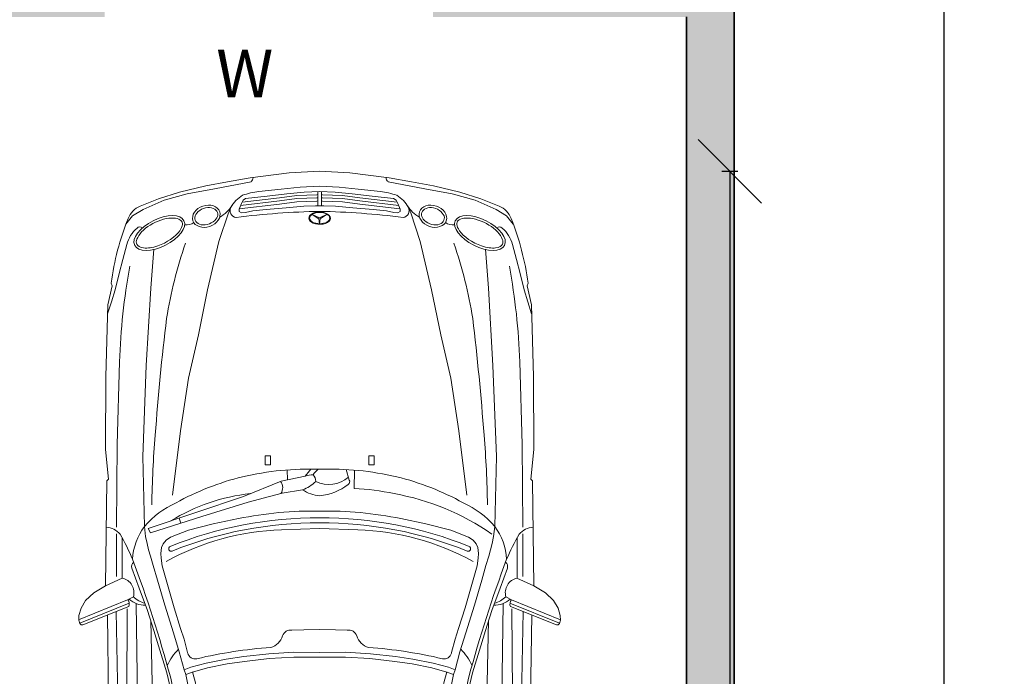
# Model space of a CAD drawing. Units: inches. Extents: x 2247 to 2713, y 588 to 1209.
# Tile 3 of 5: x 2574 to 2698, y 725 to 808. Entities that reach past the tile are written whole.
import ezdxf

# ---------------------------------------------------------------- set-up
doc = ezdxf.new("R2010")
doc.units = ezdxf.units.IN
for name, color, linetype, lineweight in [('0_Equip', 250, 'Continuous', 18), ('A-ANNO-DIMS', 2, 'Continuous', 18), ('A-ANNO-TEXT', 7, 'Continuous', 18), ('A-WALL', 7, 'Continuous', 35), ('A-WALL-PATT', 4, 'Continuous', 13)]:
    doc.layers.add(name, color=color, linetype=linetype, lineweight=lineweight)
doc.styles.get("Standard").update_dxf_attribs({"font": 'arial.ttf'})
doc.dimstyles.new('ISO-25', dxfattribs={"dimtxt": 8, "dimasz": 8, "dimexe": 1, "dimexo": 1, "dimtad": 0, "dimtih": 1, "dimtoh": 1, "dimlunit": 3, "dimtxsty": 'Standard', "dimblk": 'OBLIQUE', "dimcen": 2.5, "dimadec": 0, "dimazin": 0, "dimtfac": 1, "dimtmove": 0, "dimatfit": 3, "dimfxl": 1, "dimfxlon": 1, "dimarcsym": 0})

# ---------------------------------------------------------------- blocks, each defined once
blk = doc.blocks.new('A$C4C7B54D1')
at = {"layer": '0_Equip', "ltscale": 0.1}
for p, q in [((-1.0176, 2.6505), (-1.112, 2.6343)), ((-0.8531, 2.6707), (-1.0176, 2.6505)), ((-0.7257, 2.678), (-0.8531, 2.6707)), ((-0.7257, 2.678), (-0.5983, 2.6707)), ((-0.5983, 2.6707), (-0.4338, 2.6505)), ((-0.4338, 2.6505), (-0.3394, 2.6343)), ((-1.2037, 2.6168), (-1.3142, 2.5898)), ((-1.112, 2.6343), (-1.2037, 2.6168)), ((-1.0138, 2.6343), (-1.1673, 2.6045)), ((-0.8072, 2.6112), (-0.8877, 2.6027)), ((-0.7257, 2.6157), (-0.8072, 2.6112)), ((-0.7257, 2.6157), (-0.6441, 2.6112)), ((-0.6441, 2.6112), (-0.5636, 2.6027)), ((-0.4376, 2.6343), (-0.284, 2.6045)), ((-0.3394, 2.6343), (-0.2477, 2.6168)), ((-0.2477, 2.6168), (-0.1371, 2.5898)), ((-1.3142, 2.5898), (-1.4032, 2.5628)), ((-1.2824, 2.5829), (-1.3789, 2.557)), ((-1.1673, 2.6045), (-1.2824, 2.5829)), ((-0.8877, 2.6027), (-0.9812, 2.5937)), ((-0.5636, 2.6027), (-0.4701, 2.5937)), ((-0.284, 2.6045), (-0.1689, 2.5829)), ((-0.1689, 2.5829), (-0.0725, 2.557)), ((-0.1371, 2.5898), (-0.0481, 2.5628)), ((-1.4032, 2.5628), (-1.4801, 2.5318)), ((-1.3789, 2.557), (-1.4667, 2.5181)), ((-0.0725, 2.557), (0.0153, 2.5181)), ((-0.0481, 2.5628), (0.0288, 2.5318)), ((-1.5113, 2.4907), (-1.5393, 2.4562)), ((-1.4667, 2.5181), (-1.5113, 2.4907)), ((-1.1083, 2.5037), (-1.1486, 2.3827)), ((-0.343, 2.5037), (-0.3027, 2.3827)), ((0.0153, 2.5181), (0.06, 2.4907)), ((0.06, 2.4907), (0.0879, 2.4562)), ((-1.5353, 2.3701), (-1.5529, 2.308)), ((-1.1486, 2.3827), (-1.1961, 2.1797)), ((-0.3027, 2.3827), (-0.2552, 2.1797)), ((0.084, 2.3701), (0.1016, 2.308)), ((-1.435, 2.1869), (-1.4221, 2.3511)), ((-0.0163, 2.1869), (-0.0293, 2.3511)), ((-1.5529, 2.308), (-1.5677, 2.2486)), ((0.1016, 2.308), (0.1164, 2.2486)), ((-1.5677, 2.2486), (-1.5849, 2.1795)), ((0.1164, 2.2486), (0.1336, 2.1795)), ((-1.597, 2.1976), (-1.615, 2.1169)), ((-1.6012, 2.2082), (-1.597, 2.1976)), ((0.1499, 2.2082), (0.1457, 2.1976)), ((0.1457, 2.1976), (0.1637, 2.1169)), ((-1.5849, 2.1795), (-1.5997, 2.1304)), ((-1.4537, 1.863), (-1.435, 2.1869)), ((-1.1961, 2.1797), (-1.2349, 1.9911)), ((-0.2552, 2.1797), (-0.2164, 1.9911)), ((0.0024, 1.863), (-0.0163, 2.1869)), ((0.1336, 2.1795), (0.1484, 2.1304)), ((-1.615, 2.1169), (-1.6235, 1.8165)), ((-1.5997, 2.1304), (-1.6161, 2.0798)), ((0.1484, 2.1304), (0.1647, 2.0798)), ((0.1637, 2.1169), (0.1722, 1.8165)), ((-1.2349, 1.9911), (-1.2767, 1.8097)), ((-0.2164, 1.9911), (-0.1746, 1.8097)), ((-1.566, 1.8774), (-1.5761, 1.5304)), ((-1.4681, 1.48), (-1.4537, 1.863)), ((0.0168, 1.48), (0.0024, 1.863)), ((0.1147, 1.8774), (0.1247, 1.5304)), ((-1.6235, 1.8165), (-1.6256, 1.5098)), ((-1.2767, 1.8097), (-1.3098, 1.588)), ((-0.1746, 1.8097), (-0.1415, 1.588)), ((0.1722, 1.8165), (0.1743, 1.5098)), ((-1.3098, 1.588), (-1.3443, 1.3187)), ((-0.1415, 1.588), (-0.107, 1.3187)), ((-1.5761, 1.5304), (-1.5789, 1.1834)), ((0.1247, 1.5304), (0.1276, 1.1834)), ((-1.6256, 1.5098), (-1.6129, 1.3846)), ((0.1743, 1.5098), (0.1616, 1.3846)), ((-1.461, 1.1868), (-1.4681, 1.48)), ((-0.955, 1.4459), (-0.955, 1.4827)), ((-0.955, 1.4827), (-0.9321, 1.4827)), ((-0.9321, 1.4827), (-0.9321, 1.4459)), ((-0.5192, 1.4827), (-0.5192, 1.4459)), ((-0.4964, 1.4827), (-0.5192, 1.4827)), ((-0.4964, 1.4459), (-0.4964, 1.4827)), ((0.0097, 1.1868), (0.0168, 1.48)), ((-0.9321, 1.4459), (-0.955, 1.4459)), ((-0.8614, 1.4242), (-0.8603, 1.382)), ((-0.6135, 1.4258), (-0.6012, 1.3814)), ((-0.5809, 1.3459), (-0.5793, 1.4233)), ((-0.5192, 1.4459), (-0.4964, 1.4459)), ((-1.6193, 1.3782), (-1.6252, 0.9375)), ((-1.6129, 1.3846), (-1.6193, 1.3782)), ((-0.8878, 1.3764), (-1.0456, 1.313)), ((-0.7861, 1.3973), (-0.8878, 1.3764)), ((0.1616, 1.3846), (0.1679, 1.3782)), ((0.1679, 1.3782), (0.1739, 0.9375)), ((-0.9361, 1.3119), (-0.8835, 1.3269)), ((-0.8835, 1.3269), (-0.7975, 1.3408)), ((-1.0456, 1.313), (-1.4462, 1.1776)), ((-1.2207, 1.2292), (-1.0263, 1.2883)), ((-1.0263, 1.2883), (-0.9361, 1.3119)), ((-1.4366, 1.1604), (-1.2207, 1.2292)), ((-1.3162, 1.2215), (-1.3088, 1.2011)), ((-1.0667, 1.22), (-1.1723, 1.1976)), ((-0.3847, 1.22), (-0.279, 1.1976)), ((-1.4565, 1.1447), (-1.461, 1.1868)), ((-1.4462, 1.1776), (-1.4366, 1.1604)), ((-1.2762, 1.1716), (-1.3515, 1.142)), ((-1.1723, 1.1976), (-1.2762, 1.1716)), ((-0.7257, 1.1776), (-0.8858, 1.1725)), ((-0.7257, 1.1776), (-0.5655, 1.1725)), ((-0.279, 1.1976), (-0.1751, 1.1716)), ((-0.1751, 1.1716), (-0.0999, 1.142)), ((0.0052, 1.1447), (0.0097, 1.1868)), ((-1.5793, 1.1562), (-1.5793, 0.9761)), ((-1.5552, 1.139), (-1.5552, 0.9693)), ((-1.4503, 1.1151), (-1.4565, 1.1447)), ((-1.3703, 1.1286), (-1.3828, 1.1133)), ((-1.3515, 1.142), (-1.3703, 1.1286)), ((-0.0999, 1.142), (-0.0811, 1.1286)), ((-0.0811, 1.1286), (-0.0685, 1.1133)), ((-0.0011, 1.1151), (0.0052, 1.1447)), ((0.1038, 1.139), (0.1038, 0.9693)), ((0.128, 1.1562), (0.128, 0.9761)), ((-1.444, 1.0892), (-1.4503, 1.1151)), ((-1.4368, 1.0623), (-1.444, 1.0892)), ((-1.39, 1.0981), (-1.3927, 1.0739)), ((-1.3828, 1.1133), (-1.39, 1.0981)), ((-0.0685, 1.1133), (-0.0614, 1.0981)), ((-0.0614, 1.0981), (-0.0587, 1.0739)), ((-0.0145, 1.0623), (-0.0073, 1.0892)), ((-0.0073, 1.0892), (-0.0011, 1.1151)), ((-1.4243, 1.0229), (-1.4368, 1.0623)), ((-1.3927, 1.0739), (-1.3918, 1.0533)), ((-1.3918, 1.0533), (-1.3867, 1.0211)), ((-0.0596, 1.0533), (-0.0646, 1.0211)), ((-0.0587, 1.0739), (-0.0596, 1.0533)), ((-0.027, 1.0229), (-0.0145, 1.0623)), ((-1.5149, 1.011), (-1.4844, 0.9277)), ((-1.4064, 0.961), (-1.4243, 1.0229)), ((-1.3867, 1.0211), (-1.3374, 0.8446)), ((-0.0646, 1.0211), (-0.1139, 0.8446)), ((-0.0449, 0.961), (-0.027, 1.0229)), ((0.0635, 1.011), (0.0331, 0.9277)), ((-1.6252, 0.9375), (-1.5546, 0.9696)), ((-1.3759, 0.8562), (-1.4064, 0.961)), ((-0.0754, 0.8562), (-0.0449, 0.961)), ((0.1739, 0.9375), (0.1032, 0.9696)), ((-1.6252, 0.9375), (-1.6745, 0.908)), ((-1.4844, 0.9277), (-1.4486, 0.8345)), ((0.0331, 0.9277), (-0.0028, 0.8345)), ((0.1739, 0.9375), (0.2232, 0.908)), ((-1.5321, 0.8786), (-1.7381, 0.7945)), ((-1.7088, 0.8764), (-1.728, 0.8432)), ((-1.6745, 0.908), (-1.7088, 0.8764)), ((-1.508, 0.8914), (-1.5321, 0.8786)), ((0.0566, 0.8914), (0.0807, 0.8786)), ((0.0807, 0.8786), (0.2867, 0.7945)), ((0.2232, 0.908), (0.2574, 0.8764)), ((0.2574, 0.8764), (0.2767, 0.8432)), ((-1.728, 0.8432), (-1.7366, 0.8127)), ((-1.5253, 0.865), (-1.7329, 0.7802)), ((-1.5273, 0.8512), (-1.7203, 0.7738)), ((-1.5805, 0.8299), (-1.5623, -0.138)), ((-1.5337, 0.8406), (-1.5355, 0.484)), ((-1.4835, -0.0735), (-1.497, 0.863)), ((-1.4486, 0.8345), (-1.4226, 0.7503)), ((-1.3401, 0.7406), (-1.3759, 0.8562)), ((-1.3374, 0.8446), (-1.3097, 0.7577)), ((-0.1139, 0.8446), (-0.1417, 0.7577)), ((-0.1112, 0.7406), (-0.0754, 0.8562)), ((-0.0028, 0.8345), (-0.0287, 0.7503)), ((0.0322, -0.0735), (0.0457, 0.863)), ((0.074, 0.865), (0.2816, 0.7802)), ((0.0759, 0.8512), (0.269, 0.7738)), ((0.0824, 0.8406), (0.0842, 0.484)), ((0.1292, 0.8299), (0.111, -0.138)), ((0.2767, 0.8432), (0.2853, 0.8127)), ((-1.7366, 0.8127), (-1.7377, 0.7934)), ((-1.7377, 0.7934), (-1.7327, 0.7794)), ((-1.6171, 0.8152), (-1.5964, -0.6171)), ((-1.4352, 0.792), (-1.4152, -0.045)), ((-0.0162, 0.792), (-0.0361, -0.045)), ((0.1658, 0.8152), (0.145, -0.6171)), ((0.2863, 0.7934), (0.2813, 0.7794)), ((0.2853, 0.8127), (0.2863, 0.7934)), ((-1.4226, 0.7503), (-1.4029, 0.6849)), ((-1.3097, 0.7577), (-1.2953, 0.7129)), ((-0.7926, 0.7532), (-0.8418, 0.7514)), ((-0.7257, 0.7541), (-0.7926, 0.7532)), ((-0.7257, 0.7541), (-0.6587, 0.7532)), ((-0.6587, 0.7532), (-0.6095, 0.7514)), ((-0.1417, 0.7577), (-0.156, 0.7129)), ((-0.0287, 0.7503), (-0.0484, 0.6849)), ((-1.315, 0.66), (-1.3401, 0.7406)), ((-1.2953, 0.7129), (-1.2801, 0.6573)), ((-0.156, 0.7129), (-0.1712, 0.6573)), ((-0.1363, 0.66), (-0.1112, 0.7406)), ((-1.4029, 0.6849), (-1.368, 0.5729)), ((-0.0484, 0.6849), (-0.0834, 0.5729)), ((-1.2951, 0.5849), (-1.315, 0.66)), ((-1.2801, 0.6573), (-1.2795, 0.6546)), ((-1.1177, 0.6302), (-1.2021, 0.6133)), ((-1.0437, 0.6403), (-1.1177, 0.6302)), ((-0.9389, 0.6526), (-1.0437, 0.6403)), ((-0.937, 0.6317), (-1.0411, 0.6196)), ((-0.8346, 0.6593), (-0.9389, 0.6526)), ((-0.834, 0.6384), (-0.937, 0.6317)), ((-0.7257, 0.6582), (-0.8346, 0.6593)), ((-0.7257, 0.6373), (-0.834, 0.6384)), ((-0.7257, 0.6582), (-0.6168, 0.6593)), ((-0.7257, 0.6373), (-0.6173, 0.6384)), ((-0.6173, 0.6384), (-0.5143, 0.6317)), ((-0.6168, 0.6593), (-0.5124, 0.6526)), ((-0.5143, 0.6317), (-0.4102, 0.6196)), ((-0.5124, 0.6526), (-0.4076, 0.6403)), ((-0.4076, 0.6403), (-0.3337, 0.6302)), ((-0.3337, 0.6302), (-0.2492, 0.6133)), ((-0.1712, 0.6573), (-0.1719, 0.6546)), ((-0.1562, 0.5849), (-0.1363, 0.66)), ((-1.2663, 0.5956), (-1.2951, 0.5849)), ((-1.2879, 0.5653), (-1.2951, 0.5849)), ((-1.2021, 0.6133), (-1.2663, 0.5956)), ((-1.1973, 0.593), (-1.2599, 0.5757)), ((-1.1142, 0.6096), (-1.1973, 0.593)), ((-1.0411, 0.6196), (-1.1142, 0.6096)), ((-0.4102, 0.6196), (-0.3371, 0.6096)), ((-0.3371, 0.6096), (-0.2541, 0.593)), ((-0.2541, 0.593), (-0.1914, 0.5757)), ((-0.2492, 0.6133), (-0.185, 0.5956)), ((-0.185, 0.5956), (-0.1562, 0.5849)), ((-0.1635, 0.5653), (-0.1562, 0.5849)), ((-1.368, 0.5729), (-1.3527, 0.5066)), ((-1.2599, 0.5757), (-1.2879, 0.5653)), ((-0.1914, 0.5757), (-0.1635, 0.5653)), ((-0.0834, 0.5729), (-0.0986, 0.5066)), ((-1.3527, 0.5066), (-1.3411, 0.4394)), ((-0.0986, 0.5066), (-0.1102, 0.4394)), ((-1.5355, 0.484), (-1.5292, 0.2045)), ((0.0842, 0.484), (0.0779, 0.2045)), ((-1.3411, 0.4394), (-1.3321, 0.3749)), ((-0.1102, 0.4394), (-0.1192, 0.3749)), ((-1.3321, 0.3749), (-1.3286, 0.3301)), ((-0.7257, 0.4085), (-1.0528, 0.4085)), ((-0.7257, 0.4085), (-0.3986, 0.4085)), ((-0.1192, 0.3749), (-0.1228, 0.3301)), ((-1.3178, 0.3418), (-1.31, 0.2426)), ((-0.1335, 0.3418), (-0.1413, 0.2426)), ((-1.3286, 0.3301), (-1.3204, 0.1751)), ((-1.1468, 0.3145), (-1.1468, 0.0145)), ((-0.3045, 0.3145), (-0.3045, 0.0145)), ((-0.1228, 0.3301), (-0.1309, 0.1751)), ((-1.31, 0.2426), (-1.306, 0.1454)), ((-0.1413, 0.2426), (-0.1454, 0.1454)), ((-1.5292, 0.2045), (-1.5185, -0.0974)), ((-1.3204, 0.1751), (-1.3164, 0.0193)), ((-0.1309, 0.1751), (-0.1349, 0.0193)), ((0.0779, 0.2045), (0.0672, -0.0974)), ((-1.306, 0.1454), (-1.3036, 0.0305)), ((-0.1454, 0.1454), (-0.1478, 0.0305)), ((-1.5798, 0.0505), (-1.5879, 0.0456)), ((-1.5879, 0.0456), (-1.5863, -0.0676)), ((0.1285, 0.0505), (0.1365, 0.0456)), ((0.1365, 0.0456), (0.1349, -0.0676)), ((-1.3164, 0.0193), (-1.3178, -0.1112)), ((-1.3036, 0.0305), (-1.3044, -0.1358)), ((-0.1478, 0.0305), (-0.147, -0.1358)), ((-0.1349, 0.0193), (-0.1335, -0.1112)), ((-1.5863, -0.0676), (-1.5806, -0.0692)), ((-0.7257, -0.0796), (-1.0528, -0.0796)), ((-0.7257, -0.0796), (-0.3986, -0.0796)), ((0.1349, -0.0676), (0.1293, -0.0692)), ((-1.4948, -0.0965), (-1.5413, -0.143)), ((-1.4857, -0.1082), (-1.4866, -0.2223)), ((-1.3774, -0.0972), (-1.3178, -0.1112)), ((-0.0739, -0.0972), (-0.1335, -0.1112)), ((0.0344, -0.1082), (0.0352, -0.2223)), ((0.0435, -0.0965), (0.0899, -0.143)), ((-1.5413, -0.143), (-1.5686, -0.1663)), ((-1.5147, -0.1299), (-1.5058, -0.3725)), ((0.0633, -0.1299), (0.0545, -0.3725)), ((0.0899, -0.143), (0.1172, -0.1663)), ((-1.4713, -0.1773), (-1.4737, -0.2127)), ((0.02, -0.1773), (0.0224, -0.2127)), ((-1.4866, -0.2223), (-1.4809, -0.3653)), ((-1.4737, -0.2127), (-1.4705, -0.3187)), ((0.0224, -0.2127), (0.0192, -0.3187)), ((0.0352, -0.2223), (0.0296, -0.3653)), ((-1.3211, -0.2496), (-1.3332, -0.3629)), ((-0.1302, -0.2496), (-0.1182, -0.3629)), ((-1.4705, -0.3187), (-1.4649, -0.4424)), ((0.0192, -0.3187), (0.0135, -0.4424)), ((-1.4809, -0.3653), (-1.4745, -0.5203)), ((-1.3332, -0.3629), (-1.3516, -0.4906)), ((-0.1182, -0.3629), (-0.0997, -0.4906)), ((0.0296, -0.3653), (0.0232, -0.5203)), ((-1.5058, -0.3725), (-1.4922, -0.6007)), ((0.0545, -0.3725), (0.0408, -0.6007)), ((-1.4649, -0.4424), (-1.4576, -0.5822)), ((0.0135, -0.4424), (0.0063, -0.5822)), ((-1.3516, -0.4906), (-1.3725, -0.5902)), ((-0.0997, -0.4906), (-0.0788, -0.5902)), ((-1.4745, -0.5203), (-1.4665, -0.6617)), ((0.0232, -0.5203), (0.0151, -0.6617)), ((-1.5964, -0.6171), (-1.5863, -0.6228)), ((-1.4922, -0.6007), (-1.4712, -0.814)), ((-1.4576, -0.5822), (-1.4384, -0.7806)), ((-1.3725, -0.5902), (-1.3942, -0.6641)), ((-0.0788, -0.5902), (-0.0571, -0.6641)), ((0.0063, -0.5822), (-0.013, -0.7806)), ((0.0408, -0.6007), (0.0198, -0.814)), ((0.145, -0.6171), (0.1349, -0.6228)), ((-1.5863, -0.6228), (-1.5949, -0.6885)), ((-1.4665, -0.6617), (-1.4552, -0.7742)), ((-1.3094, -0.9936), (-1.2569, -0.6398)), ((-0.1419, -0.9936), (-0.1944, -0.6398)), ((0.0151, -0.6617), (0.0039, -0.7742)), ((0.1349, -0.6228), (0.1436, -0.6885)), ((-1.5949, -0.6885), (-1.605, -0.843)), ((-1.3942, -0.6641), (-1.4199, -0.7485)), ((-0.0571, -0.6641), (-0.0314, -0.7485)), ((0.1436, -0.6885), (0.1537, -0.843)), ((-1.2616, -0.7846), (-1.2511, -0.7134)), ((-0.1898, -0.7846), (-0.2003, -0.7134)), ((-1.4199, -0.7485), (-1.4384, -0.7806)), ((-1.2826, -0.9445), (-1.2616, -0.7846)), ((-0.9336, -0.7717), (-0.7257, -0.7787)), ((-0.9331, -0.7613), (-0.7253, -0.7683)), ((-0.5182, -0.7613), (-0.726, -0.7683)), ((-0.5177, -0.7717), (-0.7257, -0.7787)), ((-0.1688, -0.9445), (-0.1898, -0.7846)), ((-0.0314, -0.7485), (-0.013, -0.7806)), ((-1.605, -0.843), (-1.605, -1.0322)), ((0.1537, -0.843), (0.1537, -1.0322)), ((-1.3094, -1.1068), (-1.2826, -0.9445)), ((-0.1419, -1.1068), (-0.1688, -0.9445)), ((-1.605, -1.0322), (-1.592, -1.2661)), ((-1.3444, -1.2014), (-1.3094, -0.9936)), ((-0.1069, -1.2014), (-0.1419, -0.9936)), ((0.1537, -1.0322), (0.1407, -1.2661)), ((-1.3386, -1.2925), (-1.3094, -1.1068)), ((-0.1127, -1.2925), (-0.1419, -1.1068)), ((-1.565, -1.3405), (-1.592, -1.2661)), ((-1.592, -1.2661), (-1.5848, -1.3051)), ((0.1137, -1.3405), (0.1407, -1.2661)), ((0.1407, -1.2661), (0.1335, -1.3051)), ((-1.5848, -1.3051), (-1.5762, -1.4004)), ((-1.1985, -1.3182), (-1.1694, -1.3835)), ((-0.2528, -1.3182), (-0.282, -1.3835)), ((0.1335, -1.3051), (0.1248, -1.4004)), ((-1.5417, -1.4736), (-1.565, -1.3405)), ((-0.88, -1.3337), (-0.8328, -1.3271)), ((-0.8328, -1.3271), (-0.7257, -1.3271)), ((-0.6185, -1.3271), (-0.7257, -1.3271)), ((-0.5713, -1.3337), (-0.6185, -1.3271)), ((0.0904, -1.4736), (0.1137, -1.3405)), ((-1.5762, -1.4004), (-1.5486, -1.6107)), ((-1.0858, -1.3979), (-1.0181, -1.3979)), ((-0.8309, -1.402), (-0.8409, -1.4088)), ((-0.8163, -1.3979), (-0.8309, -1.402)), ((-0.7257, -1.3974), (-0.8163, -1.3979)), ((-0.7257, -1.3974), (-0.635, -1.3979)), ((-0.635, -1.3979), (-0.6204, -1.402)), ((-0.6204, -1.402), (-0.6104, -1.4088)), ((-0.3655, -1.3979), (-0.4333, -1.3979)), ((0.1248, -1.4004), (0.0973, -1.6107)), ((-0.8664, -1.4423), (-0.8696, -1.4545)), ((-0.861, -1.4312), (-0.8664, -1.4423)), ((-0.8558, -1.4236), (-0.861, -1.4312)), ((-0.8488, -1.4158), (-0.8558, -1.4236)), ((-0.8409, -1.4088), (-0.8488, -1.4158)), ((-0.6104, -1.4088), (-0.6025, -1.4158)), ((-0.6025, -1.4158), (-0.5955, -1.4236)), ((-0.5955, -1.4236), (-0.5904, -1.4312)), ((-0.5904, -1.4312), (-0.585, -1.4423)), ((-0.585, -1.4423), (-0.5817, -1.4545)), ((-1.4962, -1.7129), (-1.5417, -1.4736)), ((-1.0923, -1.4501), (-0.9989, -1.4699)), ((-0.9989, -1.4699), (-0.8846, -1.4828)), ((-0.8807, -1.4821), (-0.8846, -1.4828)), ((-0.8846, -1.4828), (-0.8799, -1.5038)), ((-0.8769, -1.4791), (-0.8807, -1.4821)), ((-0.8745, -1.477), (-0.8769, -1.4791)), ((-0.8731, -1.467), (-0.8745, -1.477)), ((-0.8696, -1.4545), (-0.8731, -1.467)), ((-0.7257, -1.4865), (-0.8374, -1.4884)), ((-0.7257, -1.4865), (-0.6139, -1.4884)), ((-0.5817, -1.4545), (-0.5782, -1.467)), ((-0.5782, -1.467), (-0.5768, -1.477)), ((-0.5768, -1.477), (-0.5744, -1.4791)), ((-0.5744, -1.4791), (-0.5706, -1.4821)), ((-0.5668, -1.4828), (-0.5714, -1.5038)), ((-0.5706, -1.4821), (-0.5668, -1.4828)), ((-0.4524, -1.4699), (-0.5668, -1.4828)), ((-0.359, -1.4501), (-0.4524, -1.4699)), ((0.0448, -1.7129), (0.0904, -1.4736)), ((-1.3456, -1.5004), (-1.3433, -1.7188)), ((-0.8799, -1.5038), (-0.8706, -1.5038)), ((-0.7257, -1.4969), (-0.837, -1.4988)), ((-0.7257, -1.4969), (-0.6143, -1.4988)), ((-0.5714, -1.5038), (-0.5808, -1.5038)), ((-0.1057, -1.5004), (-0.1081, -1.7188)), ((-0.8799, -1.5352), (-0.7257, -1.5393)), ((-0.5714, -1.5352), (-0.7257, -1.5393)), ((-1.5486, -1.6107), (-1.5024, -1.8663)), ((-0.8502, -1.5951), (-0.7257, -1.5951)), ((-0.6011, -1.5951), (-0.7257, -1.5951)), ((0.0973, -1.6107), (0.0511, -1.8663)), ((-0.8507, -1.616), (-0.7257, -1.616)), ((-0.6006, -1.616), (-0.7257, -1.616)), ((-1.4584, -1.8701), (-1.4962, -1.7129)), ((-1.3433, -1.7188), (-1.3304, -1.8962)), ((-0.1081, -1.7188), (-0.1209, -1.8962)), ((0.0071, -1.8701), (0.0448, -1.7129)), ((-1.5024, -1.8663), (-1.4894, -1.914)), ((0.0511, -1.8663), (0.0381, -1.914)), ((-1.2767, -1.9721), (-1.3526, -1.9616)), ((-1.1845, -1.9838), (-1.2767, -1.9721)), ((-1.055, -1.9908), (-1.1845, -1.9838)), ((-1.055, -1.9768), (-1.055, -1.9908)), ((-0.7257, -1.985), (-1.055, -1.9768)), ((-0.7257, -1.985), (-0.3964, -1.9768)), ((-0.3964, -1.9768), (-0.3964, -1.9908)), ((-0.3964, -1.9908), (-0.2668, -1.9838)), ((-0.2668, -1.9838), (-0.1746, -1.9721)), ((-0.1746, -1.9721), (-0.0987, -1.9616)), ((-1.3797, -2.0208), (-1.1314, -2.0483)), ((-0.9663, -2.0048), (-0.7257, -2.0048)), ((-0.4851, -2.0048), (-0.7257, -2.0048)), ((-0.0716, -2.0208), (-0.3199, -2.0483)), ((-1.1314, -2.0483), (-0.8803, -2.0598)), ((-1.0585, -2.0375), (-0.9383, -2.0469)), ((-0.9383, -2.0469), (-0.7784, -2.0504)), ((-0.8803, -2.0598), (-0.7257, -2.0598)), ((-0.7784, -2.0504), (-0.7257, -2.0504)), ((-0.673, -2.0504), (-0.7257, -2.0504)), ((-0.5711, -2.0598), (-0.7257, -2.0598)), ((-0.5131, -2.0469), (-0.673, -2.0504)), ((-0.3199, -2.0483), (-0.5711, -2.0598)), ((-0.3929, -2.0375), (-0.5131, -2.0469))]:
    blk.add_line(p, q, dxfattribs=at)
at = {"layer": '0_Equip'}
for p, q in [((-1.0517, 2.5482), (-0.8949, 2.567)), ((-0.9467, 2.5739), (-1.0364, 2.5634)), ((-0.8628, 2.5838), (-0.9467, 2.5739)), ((-0.8949, 2.567), (-0.8211, 2.5763)), ((-0.7905, 2.5897), (-0.8628, 2.5838)), ((-0.8211, 2.5763), (-0.738, 2.5791)), ((-0.8211, 2.5631), (-0.738, 2.5659)), ((-0.7257, 2.5926), (-0.7905, 2.5897)), ((-0.738, 2.5791), (-0.733, 2.58)), ((-0.738, 2.5659), (-0.733, 2.5668)), ((-0.733, 2.5923), (-0.733, 2.5325)), ((-0.7257, 2.5926), (-0.6608, 2.5897)), ((-0.7183, 2.5923), (-0.7183, 2.5325)), ((-0.7133, 2.5791), (-0.7183, 2.58)), ((-0.7133, 2.5659), (-0.7183, 2.5668)), ((-0.6302, 2.5763), (-0.7133, 2.5791)), ((-0.6302, 2.5631), (-0.7133, 2.5659)), ((-0.6608, 2.5897), (-0.5886, 2.5838)), ((-0.5564, 2.567), (-0.6302, 2.5763)), ((-0.5886, 2.5838), (-0.5046, 2.5739)), ((-0.3996, 2.5482), (-0.5564, 2.567)), ((-0.5046, 2.5739), (-0.4149, 2.5634)), ((-1.0545, 2.5425), (-1.0638, 2.5185)), ((-1.0631, 2.5204), (-0.8949, 2.5405)), ((-1.0577, 2.5343), (-0.8949, 2.5537)), ((-1.0475, 2.557), (-1.0545, 2.5425)), ((-1.0364, 2.5634), (-1.0475, 2.557)), ((-0.9502, 2.5168), (-0.8657, 2.5238)), ((-0.8949, 2.5537), (-0.8211, 2.5631)), ((-0.8949, 2.5405), (-0.8211, 2.5498)), ((-0.8657, 2.5238), (-0.7922, 2.5308)), ((-0.8211, 2.5498), (-0.738, 2.5526)), ((-0.7922, 2.5308), (-0.7433, 2.5325)), ((-0.7433, 2.5325), (-0.7257, 2.5325)), ((-0.738, 2.5526), (-0.733, 2.5536)), ((-0.708, 2.5325), (-0.7257, 2.5325)), ((-0.7133, 2.5526), (-0.7183, 2.5536)), ((-0.6302, 2.5498), (-0.7133, 2.5526)), ((-0.6591, 2.5308), (-0.708, 2.5325)), ((-0.5857, 2.5238), (-0.6591, 2.5308)), ((-0.5564, 2.5537), (-0.6302, 2.5631)), ((-0.5564, 2.5405), (-0.6302, 2.5498)), ((-0.5011, 2.5168), (-0.5857, 2.5238)), ((-0.3936, 2.5343), (-0.5564, 2.5537)), ((-0.3882, 2.5204), (-0.5564, 2.5405)), ((-0.4149, 2.5634), (-0.4038, 2.557)), ((-0.4038, 2.557), (-0.3968, 2.5425)), ((-0.3968, 2.5425), (-0.3875, 2.5185)), ((-1.0638, 2.5185), (-1.0638, 2.5092)), ((-1.0638, 2.5092), (-1.0545, 2.504)), ((-1.0545, 2.504), (-1.0376, 2.5051)), ((-1.0376, 2.5051), (-1.0067, 2.5116)), ((-1.0067, 2.5116), (-0.9502, 2.5168)), ((-0.7566, 2.4971), (-0.7261, 2.4828)), ((-0.7566, 2.4971), (-0.7291, 2.4776)), ((-0.7389, 2.5095), (-0.7395, 2.5059)), ((-0.6947, 2.4974), (-0.7261, 2.4828)), ((-0.6947, 2.4974), (-0.723, 2.4776)), ((-0.7124, 2.5095), (-0.7119, 2.5059)), ((-0.4446, 2.5116), (-0.5011, 2.5168)), ((-0.4137, 2.5051), (-0.4446, 2.5116)), ((-0.3968, 2.504), (-0.4137, 2.5051)), ((-0.3875, 2.5092), (-0.3968, 2.504)), ((-0.3875, 2.5185), (-0.3875, 2.5092)), ((-0.7259, 2.4578), (-0.7291, 2.4776)), ((-0.7259, 2.4578), (-0.723, 2.4776))]:
    blk.add_line(p, q, dxfattribs=at)
at = {"layer": '0_Equip', "ltscale": 0.1}
for centre in [(-1.4513, 0), (0, 0)]:
    blk.add_circle(centre, 0.00662, dxfattribs=at)
for centre, radius, start, end in [((-1.0252, 2.6508), 0.02, 304.7228, 3.5172), ((-0.4261, 2.6508), 0.02, 176.4828, 235.2772), ((-0.9799, 2.461), 0.1353, 120.8369, 151.2853), ((-0.9299, 2.2354), 0.3619, 98.1466, 109.2524), ((-0.5214, 2.2354), 0.3619, 70.7476, 81.8534), ((-0.4714, 2.461), 0.1353, 28.7147, 59.1631), ((-1.4391, 2.4422), 0.0986, 114.5945, 157.5113), ((-1.2153, 2.6098), 0.1432, 299.1564, 328.1831), ((-0.9799, 2.461), 0.1353, 151.2853, 161.5889), ((-1.0728, 2.5126), 0.029, 152.6038, 261.721), ((-0.3785, 2.5126), 0.029, 278.279, 27.3962), ((-0.236, 2.6098), 0.1432, 211.8169, 240.8436), ((-0.4714, 2.461), 0.1353, 18.4111, 28.7147), ((-0.0123, 2.4422), 0.0986, 22.4887, 65.4055), ((-0.6679, -0.6671), 3.1773, 91.0415, 97.3969), ((-0.7834, -0.6671), 3.1773, 82.6031, 88.9585), ((-0.4722, 2.0579), 1.139, 158.2564, 172.4203), ((-1.4798, 2.4259), 0.0184, 54.8052, 134.0204), ((-1.2841, 2.5028), 0.0501, 260.5448, 306.7068), ((-0.1672, 2.5028), 0.0501, 233.2932, 279.4552), ((0.0285, 2.4259), 0.0184, 45.9796, 125.1948), ((-0.9791, 2.0579), 1.139, 7.5797, 21.7436), ((-1.4083, 2.3394), 0.1306, 130.2084, 166.4224), ((-0.043, 2.3394), 0.1306, 13.5776, 49.7916), ((0.5502, 1.746), 1.9445, 161.1117, 170.7019), ((-2.0015, 1.746), 1.9445, 9.2981, 18.8883), ((1.1202, 1.7918), 2.6875, 169.5541, 178.1755), ((-2.5715, 1.7918), 2.6875, 1.8245, 10.4459), ((9.2655, 0.7813), 10.7109, 173.14258, 175.77374), ((-10.7169, 0.7813), 10.7109, 4.22626, 6.85742), ((2.9623, 1.2089), 4.3935, 175.2767, 179.1124), ((-4.4136, 1.2089), 4.3935, 0.8876, 4.7233), ((-0.7686, 0.201), 1.2267, 87.9955, 103.2364), ((-0.3726, 1.0935), 0.5131, 139.3585, 143.6922), ((-0.6528, 1.3354), 0.1211, 130.7679, 145.6911), ((-0.6828, 0.201), 1.2267, 76.7636, 92.0045), ((-0.786, 0.3109), 1.1158, 103.6551, 119.1148), ((-0.9216, 1.3498), 0.0409, 323.4512, 39.0343), ((-0.8494, 1.486), 0.1542, 289.6676, 314.192), ((-0.7554, 1.327), 0.0768, 88.1186, 113.6019), ((-0.7803, 1.3768), 0.0384, 357.9275, 44.3829), ((-0.6872, 1.4869), 0.1241, 243.8649, 311.6638), ((-0.6113, 1.3746), 0.0122, 294.8678, 33.6398), ((-0.6653, 0.3109), 1.1158, 60.8852, 76.3449), ((-0.929, 0.5266), 0.803, 96.22, 121.6991), ((-0.7147, 1.4628), 0.1474, 235.8143, 265.7174), ((-0.741, 1.5272), 0.212, 274.1513, 309.4931), ((-0.617, 0.3882), 0.9584, 77.6919, 87.8428), ((-0.5976, 0.2949), 1.0461, 55.3038, 79.8165), ((-1.1803, 0.9494), 0.3676, 113.8511, 139.7847), ((-0.2711, 0.9494), 0.3676, 40.2153, 66.1489), ((-0.7478, -0.378), 1.6295, 89.2231, 101.2856), ((-0.7036, -0.378), 1.6295, 78.7144, 90.7769), ((-0.7356, -0.4312), 1.6538, 89.6554, 111.9286), ((-0.7356, -0.4312), 1.6329, 89.6554, 111.9286), ((-0.7157, -0.4312), 1.6538, 68.0714, 90.3446), ((-0.7157, -0.4312), 1.6329, 68.0714, 90.3446), ((-1.6261, 1.102), 0.0813, 40.278, 87.0689), ((-1.2706, 1.0395), 0.2408, 142.2718, 177.7746), ((-0.85, 0.0855), 1.0875, 91.8892, 118.6013), ((-0.6014, 0.0855), 1.0875, 61.3987, 88.1108), ((-0.1807, 1.0395), 0.2408, 2.2254, 37.7282), ((0.1747, 1.102), 0.0813, 92.9311, 139.722), ((-2.3477, 0.6968), 0.9076, 22.824, 30.2904), ((0.8964, 0.6968), 0.9076, 149.7096, 157.176), ((-1.3493, 1.0932), 0.0105, 111.9286, 291.9286), ((-0.102, 1.0932), 0.0105, 248.0714, 68.0714), ((-1.4887, 1.0171), 0.0269, 132.3277, 193.1064), ((-6.6059, -0.8606), 5.4408, 15.0904, 20.5451), ((5.1546, -0.8606), 5.4408, 159.4549, 164.9096), ((0.0373, 1.0171), 0.0269, 346.8936, 47.6723), ((-1.5684, 0.9084), 0.0628, 344.3283, 77.2348), ((0.1171, 0.9084), 0.0628, 102.7652, 195.6717), ((-1.5495, 0.8614), 0.0245, 335.4987, 44.5114), ((-1.463, 0.9441), 0.0879, 224.7932, 273.9292), ((-1.4233, 0.9849), 0.1262, 227.8287, 253.081), ((0.0117, 0.9441), 0.0879, 266.0708, 315.2068), ((-0.0281, 0.9849), 0.1262, 286.919, 312.1713), ((0.0982, 0.8614), 0.0245, 135.4886, 204.5013), ((-1.7238, 0.7825), 0.00941, 199.646, 291.8616), ((-0.8474, 0.7163), 0.0355, 80.937, 162.15), ((-0.6039, 0.7163), 0.0355, 17.85, 99.063), ((0.2725, 0.7825), 0.00941, 248.1384, 340.354), ((-0.9515, 0.7495), 0.0737, 286.567, 342.4011), ((-0.4998, 0.7495), 0.0737, 197.5989, 253.433), ((-1.1535, 0.5061), 0.2334, 134.9877, 155.4049), ((-0.7896, -1.2957), 1.9795, 94.0807, 103.2045), ((-0.6617, -1.2957), 1.9795, 76.7955, 85.9193), ((-0.2978, 0.5061), 0.2334, 24.5951, 45.0123), ((-1.249, 0.662), 0.0314, 193.667, 283.2045), ((-0.2023, 0.662), 0.0314, 256.7955, 346.333), ((-2.6334, 0.2371), 1.3197, 4.5498, 13.9797), ((-4.2099, -0.0242), 2.9809, 358.1905, 11.4064), ((-2.0025, 0.3511), 0.7759, 4.7259, 16.8296), ((2.7585, -0.0242), 2.9809, 168.5936, 181.8095), ((0.5512, 0.3511), 0.7759, 163.1704, 175.2741), ((1.1821, 0.2371), 1.3197, 166.0203, 175.4502), ((-1.2324, 0.3484), 0.1397, 106.6168, 134.6647), ((-0.2189, 0.3484), 0.1397, 45.3353, 73.3832), ((-6.5594, -0.126), 5.3575, 1.3159, 5.7952), ((5.1081, -0.126), 5.3575, 174.2048, 178.6841), ((-1.0528, 0.3145), 0.0941, 90, 180), ((-0.3986, 0.3145), 0.0941, 0, 90), ((-1.0944, -0.0222), 0.5055, 165.8807, 194.1193), ((-1.3066, 0.102), 0.2781, 180.1936, 190.6834), ((-1.4634, 0.1296), 0.0534, 245.2796, 326.9469), ((0.0121, 0.1296), 0.0534, 213.0531, 294.7204), ((-0.1448, 0.102), 0.2781, 349.3166, 359.8064), ((-0.3569, -0.0222), 0.5055, 345.8807, 14.1193), ((-1.7275, -0.0084), 0.159, 337.4976, 21.7335), ((0.2762, -0.0084), 0.159, 158.2665, 202.5024), ((-1.0528, 0.0145), 0.0941, 180, 270), ((-0.3986, 0.0145), 0.0941, 270, 0), ((-6.573, -0.0941), 5.3705, 356.0501, 0.9723), ((5.1217, -0.0941), 5.3705, 179.0277, 183.9499), ((-1.7817, -0.0969), 0.2029, 346.1346, 7.8419), ((-1.4831, 0.0214), 0.095, 269.7172, 315.6185), ((-1.2968, 0.3651), 0.4767, 246.9385, 267.4714), ((-1.3634, -0.0473), 0.0519, 177.4537, 254.2676), ((-0.1545, 0.3651), 0.4767, 272.5286, 293.0615), ((-0.0879, -0.0473), 0.0519, 285.7324, 2.5463), ((0.0317, 0.0214), 0.095, 224.3815, 270.2828), ((0.3303, -0.0969), 0.2029, 172.1581, 193.8654), ((-1.4874, -0.1039), 0.0105, 68.8598, 135.0096), ((-1.2476, 0.5164), 0.6547, 248.8598, 265.0222), ((-8.0298, -0.0355), 6.7998, 354.90123, 359.30214), ((6.5785, -0.0355), 6.7998, 180.69786, 185.09877), ((-0.2038, 0.5164), 0.6547, 274.9778, 291.1402), ((0.0361, -0.1039), 0.0105, 44.9904, 111.1402), ((-1.5869, -0.1514), 0.0236, 227.2909, 320.7388), ((-1.3362, 0.3542), 0.5484, 255.7347, 268.4072), ((-1.3699, -0.2402), 0.0497, 349.0381, 68.1064), ((-1.3526, -0.2358), 0.0418, 357.143, 88.4072), ((-0.0988, -0.2358), 0.0418, 91.5928, 182.857), ((-0.0814, -0.2402), 0.0497, 111.8936, 190.9619), ((-0.1152, 0.3542), 0.5484, 271.5928, 284.2653), ((0.1355, -0.1514), 0.0236, 219.2612, 312.7091), ((-3.2483, -0.1412), 1.9399, 339.54, 357.143), ((1.797, -0.1412), 1.9399, 182.857, 200.46), ((-2.454, -0.4173), 1.2396, 346.6558, 357.8401), ((1.0027, -0.4173), 1.2396, 182.1599, 193.3442), ((-0.8588, 0.5276), 1.3014, 252.4566, 266.7043), ((-0.8588, 0.5276), 1.291, 252.4566, 266.6988), ((-0.5926, 0.5276), 1.291, 273.3012, 287.5434), ((-0.5926, 0.5276), 1.3014, 273.2957, 287.5434), ((-1.1971, -0.7899), 0.0105, 79.1189, 173.1671), ((-0.7142, 1.7227), 2.5481, 259.1189, 269.7413), ((-0.7372, 1.7227), 2.5481, 270.2587, 280.8811), ((-0.2542, -0.7899), 0.0105, 6.8329, 100.8811), ((-1.4504, -0.812), 0.0209, 185.6259, 339.54), ((-5.088, -0.3237), 3.9082, 348.7726, 353.1671), ((3.6366, -0.3237), 3.9082, 186.8329, 191.2274), ((-0.001, -0.812), 0.0209, 200.46, 354.3741), ((0.625, -1.1812), 0.5281, 165.7822, 187.813), ((0.1224, -1.0639), 0.0155, 11.61, 127.0083), ((-0.7003, -1.1122), 0.8395, 350.5693, 3.5107), ((-4.7286, -0.6026), 3.5073, 348.8701, 352.1003), ((3.2772, -0.6026), 3.5073, 187.8997, 191.1299), ((-0.8187, -1.3185), 0.5386, 167.4447, 180.7102), ((-1.3591, -1.3822), 0.1728, 21.7432, 61.9432), ((-0.0922, -1.3822), 0.1728, 118.0568, 158.2568), ((-0.6326, -1.3185), 0.5386, 359.2898, 12.5553), ((-1.0952, -1.3051), 0.1937, 172.4314, 224.4267), ((-0.3561, -1.3051), 0.1937, 315.5733, 7.5686), ((0.1138, -1.243), 0.0156, 219.7819, 334.4738), ((-1.0611, -1.2979), 0.2775, 178.8811, 209.7062), ((-0.3902, -1.2979), 0.2775, 330.2938, 1.1189), ((-1.0944, -1.3104), 0.2633, 183.2136, 211.504), ((-1.0482, -1.2146), 0.1871, 220.4031, 258.3959), ((-1.0495, -1.2507), 0.1505, 282.0448, 314.7653), ((-0.8301, -1.5634), 0.235, 102.268, 118.8572), ((-0.6213, -1.5634), 0.235, 61.1428, 77.732), ((-0.4019, -1.2507), 0.1505, 225.2347, 257.9552), ((-0.4032, -1.2146), 0.1871, 281.6041, 319.5969), ((-0.3569, -1.3104), 0.2633, 328.496, 356.7864), ((-1.0421, -1.3141), 0.145, 208.6187, 249.7318), ((-0.4092, -1.3141), 0.145, 290.2682, 331.3813), ((-1.052, -1.2472), 0.313, 216.9484, 253.2054), ((-0.8912, -0.9022), 0.6331, 235.8724, 271.0227), ((-1.0459, -1.2776), 0.2487, 221.0065, 261.6946), ((-0.5601, -0.9022), 0.6331, 268.9773, 304.1276), ((-0.4054, -1.2776), 0.2487, 278.3054, 318.9935), ((-0.3993, -1.2472), 0.313, 286.7946, 323.0516), ((-1.2501, -1.516), 0.0967, 135.2951, 170.7274), ((-1.052, -1.2472), 0.3339, 216.9484, 253.2314), ((-0.8344, -1.538), 0.0498, 93.4455, 136.5439), ((-0.6169, -1.538), 0.0498, 43.4561, 86.5545), ((-0.3993, -1.2472), 0.3339, 286.7686, 323.0516), ((-0.2012, -1.516), 0.0967, 9.2726, 44.7049), ((-0.7003, 0.2815), 1.8451, 258.0669, 269.2129), ((-0.8066, -1.54), 0.0735, 150.5285, 176.2825), ((-0.8066, -1.54), 0.063, 151.7195, 175.9212), ((-0.8344, -1.538), 0.0393, 93.7549, 134.7116), ((-0.751, 0.2815), 1.8451, 270.7871, 281.9331), ((-0.6169, -1.538), 0.0393, 45.2884, 86.2451), ((-0.6447, -1.54), 0.063, 4.0788, 28.2805), ((-0.6447, -1.54), 0.0735, 3.7175, 29.4715), ((-0.7884, -0.3101), 1.3074, 254.0198, 267.2681), ((-0.7884, -0.3101), 1.2865, 254.0263, 267.246), ((-0.6629, -0.3101), 1.2865, 272.754, 285.9737), ((-0.6629, -0.3101), 1.3074, 272.7319, 285.9802), ((-1.3393, -1.8393), 0.123, 194.4986, 263.7836), ((-0.5134, 7.9307), 9.8503, 265.23745, 268.76503), ((-1.2452, -1.8915), 0.0853, 183.2055, 252.6405), ((-0.938, 7.9307), 9.8503, 271.23497, 274.76255), ((-0.2061, -1.8915), 0.0853, 287.3595, 356.7945), ((-0.1121, -1.8393), 0.123, 276.2164, 345.5014), ((-1.3628, -1.8937), 0.1282, 189.093, 262.4153), ((-0.0885, -1.8937), 0.1282, 277.5847, 350.907), ((-1.0413, -1.8225), 0.2157, 228.406, 265.4391), ((-0.41, -1.8225), 0.2157, 274.5609, 311.594), ((-0.896, -1.272), 0.7362, 257.5275, 264.5209), ((-0.5554, -1.272), 0.7362, 275.4791, 282.4725)]:
    blk.add_arc(centre, radius, start, end, dxfattribs=at)
for centre, major_axis, ratio in [((-1.2016, 2.4892), (0.0562, 0.0189), 0.759763), ((-1.399, 2.4187), (-0.1036, -0.0518), 0.497493)]:
    blk.add_ellipse(centre, major_axis=major_axis, ratio=ratio, dxfattribs=at)
at = {"layer": '0_Equip', "ltscale": 0.1, "extrusion": (0, 0, -1)}
for centre, major_axis, ratio in [((-0.2497, 2.4892), (-0.0562, 0.0189), 0.759763), ((-0.0523, 2.4187), (0.1036, -0.0518), 0.497493)]:
    blk.add_ellipse(centre, major_axis=major_axis, ratio=ratio, dxfattribs=at)
at = {"layer": '0_Equip'}
blk.add_ellipse((-0.7253, 2.4812), major_axis=(-0.0426, 0), ratio=0.550187, dxfattribs=at)
at = {"layer": '0_Equip', "ltscale": 0.1}
for points, knots in [([(-1.1548, 2.5048), (-1.1596, 2.5191), (-1.1811, 2.5294), (-1.2283, 2.5198), (-1.248, 2.5001), (-1.2511, 2.4679), (-1.2373, 2.4539), (-1.1922, 2.4512), (-1.1656, 2.4658), (-1.1532, 2.4906), (-1.1526, 2.4983), (-1.1548, 2.5048)], [0, 0, 0, 0, 1.408119, 1.408119, 2.816238, 2.816238, 4.224358, 4.224358, 5.632477, 5.632477, 6.283185, 6.283185, 6.283185, 6.283185]), ([(-0.2965, 2.5048), (-0.2917, 2.5191), (-0.2703, 2.5294), (-0.2231, 2.5198), (-0.2033, 2.5001), (-0.2003, 2.4679), (-0.2141, 2.4539), (-0.2592, 2.4512), (-0.2858, 2.4658), (-0.2981, 2.4906), (-0.2987, 2.4983), (-0.2965, 2.5048)], [0, 0, 0, 0, 1.408119, 1.408119, 2.816238, 2.816238, 4.224358, 4.224358, 5.632477, 5.632477, 6.283185, 6.283185, 6.283185, 6.283185]), ([(-1.4937, 2.3714), (-1.4901, 2.3641), (-1.4809, 2.3581), (-1.4492, 2.3543), (-1.4277, 2.3571), (-1.3679, 2.3771), (-1.3298, 2.404), (-1.2994, 2.4483), (-1.2993, 2.4626), (-1.3171, 2.4801), (-1.3406, 2.4849), (-1.3989, 2.4733), (-1.4323, 2.4577), (-1.4816, 2.4186), (-1.4956, 2.3954), (-1.4959, 2.3774), (-1.4951, 2.3742), (-1.4937, 2.3714)], [0, 0, 0, 0, 0.646556, 0.646556, 1.293113, 1.293113, 2.410172, 2.410172, 3.309931, 3.309931, 4.20969, 4.20969, 5.109449, 5.109449, 6.031285, 6.031285, 6.283185, 6.283185, 6.283185, 6.283185]), ([(0.0424, 2.3714), (0.0388, 2.3641), (0.0295, 2.3581), (-0.0022, 2.3543), (-0.0236, 2.3571), (-0.0834, 2.3771), (-0.1216, 2.404), (-0.152, 2.4483), (-0.152, 2.4626), (-0.1343, 2.4801), (-0.1108, 2.4849), (-0.0524, 2.4733), (-0.019, 2.4577), (0.0303, 2.4186), (0.0443, 2.3954), (0.0445, 2.3774), (0.0438, 2.3742), (0.0424, 2.3714)], [0, 0, 0, 0, 0.646556, 0.646556, 1.293113, 1.293113, 2.410172, 2.410172, 3.309931, 3.309931, 4.20969, 4.20969, 5.109449, 5.109449, 6.031285, 6.031285, 6.283185, 6.283185, 6.283185, 6.283185])]:
    blk.add_open_spline(points, degree=3, knots=knots, dxfattribs=at)
at = {"layer": '0_Equip'}
blk.add_open_spline([(-0.7708, 2.4812), (-0.7708, 2.4725), (-0.7635, 2.4648), (-0.7294, 2.4499), (-0.6897, 2.4563), (-0.6733, 2.4916), (-0.7036, 2.5102), (-0.7526, 2.5051), (-0.7708, 2.4948), (-0.7708, 2.4812)], degree=3, knots=[0, 0, 0, 0, 0.903923, 0.903923, 2.878844, 2.878844, 4.872977, 4.872977, 6.283185, 6.283185, 6.283185, 6.283185], dxfattribs=at)
blk = doc.blocks.new('_Oblique')
at = {"color": 0, "linetype": 'ByBlock', "lineweight": -2}
blk.add_line((-0.5, -0.5), (0.5, 0.5), dxfattribs=at)
blk = doc.blocks.new('*D12')
at = {"layer": 'A-ANNO-DIMS', "color": 0, "lineweight": -2, "transparency": 16777216}
for p, q in [((2689.46, 1168.28), (2691.46, 1168.28)), ((2690.46, 1168.28), (2690.46, 902.97)), ((2690.46, 628.28), (2690.46, 893.59)), ((2689.46, 628.28), (2691.46, 628.28))]:
    blk.add_line(p, q, dxfattribs=at)
at = {"layer": 'Defpoints', "color": 0, "transparency": 16777216}
for p in [(2664.08, 1168.28), (2664.08, 628.28), (2690.46, 628.28)]:
    blk.add_point(p, dxfattribs=at)
at = {"layer": 'A-ANNO-DIMS', "color": 0, "lineweight": -2, "transparency": 16777216, "xscale": 8, "yscale": 8, "zscale": 8}
for p, rotation in [((2690.46, 1168.28), 90), ((2690.46, 628.28), 270)]:
    blk.add_blockref('_Oblique', p, dxfattribs=dict(at, rotation=rotation))
at = {"layer": 'A-ANNO-DIMS', "color": 0, "transparency": 16777216, "insert": (2690.46, 898.28), "char_height": 8, "attachment_point": 5}
blk.add_mtext("45'", dxfattribs=at)
blk = doc.blocks.new('*D23')
at = {"layer": 'A-ANNO-DIMS', "color": 0, "lineweight": -2, "transparency": 16777216}
for p, q in [((2662.52, 788.89), (2664.52, 788.89)), ((2663.52, 788.89), (2663.52, 722.74)), ((2663.52, 647.07), (2663.52, 713.22)), ((2662.52, 647.07), (2664.52, 647.07))]:
    blk.add_line(p, q, dxfattribs=at)
at = {"layer": 'Defpoints', "color": 0, "transparency": 16777216}
for p in [(2642.25, 788.89), (2663.52, 788.89), (2642.25, 647.07)]:
    blk.add_point(p, dxfattribs=at)
at = {"layer": 'A-ANNO-DIMS', "color": 0, "lineweight": -2, "transparency": 16777216, "xscale": 8, "yscale": 8, "zscale": 8}
for p, rotation in [((2663.52, 788.89), 90), ((2663.52, 647.07), 270)]:
    blk.add_blockref('_Oblique', p, dxfattribs=dict(at, rotation=rotation))
at = {"layer": 'A-ANNO-DIMS', "color": 0, "transparency": 16777216, "insert": (2663.52, 717.98), "char_height": 8, "attachment_point": 5}
blk.add_mtext('CAR 11\'-10"', dxfattribs=at)

msp = doc.modelspace()

# ---------------------------------------------------------------- hatches: boundary and pattern name
at = {"layer": 'A-WALL-PATT'}
h = msp.add_hatch(color=256, dxfattribs=at)
h.dxf.hatch_style = 1
h.paths.add_polyline_path([(2604.041, 1168.28), (2423.716, 1168.28), (2423.716, 1162.28), (2442.076, 1162.28), (2442.076, 1114.28), (2439.021, 1114.28), (2439.021, 1108.28), (2456.056, 1108.28), (2456.056, 1114.28), (2448.076, 1114.28), (2448.076, 1162.28), (2580.076, 1162.28), (2580.076, 1114.28), (2560.507, 1114.28), (2560.507, 1108.28), (2619.195, 1108.28), (2619.195, 1114.28), (2586.076, 1114.28), (2586.076, 1162.28), (2604.041, 1162.28)])
h.paths.add_polyline_path([(2380.833, 1168.28), (2364.076, 1168.28), (2364.076, 1094.128), (2370.076, 1094.128), (2370.076, 1108.28), (2407.021, 1108.28), (2407.021, 1114.28), (2370.076, 1114.28), (2370.076, 1162.28), (2380.833, 1162.28)])
h.paths.add_polyline_path([(2664.076, 1168.28), (2639.393, 1168.28), (2639.393, 1162.28), (2658.076, 1162.28), (2658.076, 1114.28), (2651.195, 1114.28), (2651.195, 1108.28), (2658.076, 1108.28), (2658.076, 1094.128), (2664.076, 1094.128)])
h.paths.add_polyline_path([(2524.66, 1114.28), (2487.371, 1114.28), (2487.371, 1108.28), (2511.076, 1108.28), (2511.076, 940.28), (2508.076, 940.28), (2508.076, 934.28), (2520.076, 934.28), (2520.076, 940.28), (2517.076, 940.28), (2517.076, 1108.28), (2524.66, 1108.28)])
h.paths.add_polyline_path([(2370.076, 1054.172), (2364.076, 1054.172), (2364.076, 990.686), (2370.076, 990.686)])
h.paths.add_polyline_path([(2370.076, 934.28), (2472.076, 934.28), (2472.076, 940.28), (2370.076, 940.28), (2370.076, 950.99), (2364.076, 950.99), (2364.076, 902.687), (2370.076, 902.687)])
h.paths.add_polyline_path([(2664.076, 950.99), (2658.076, 950.99), (2658.076, 940.28), (2556.076, 940.28), (2556.076, 934.28), (2658.076, 934.28), (2658.076, 913.24), (2664.076, 913.24)])
h.paths.add_polyline_path([(2664.076, 1054.172), (2658.076, 1054.172), (2658.076, 990.686), (2664.076, 990.686)])
h.paths.add_polyline_path([(2664.076, 861.585), (2658.076, 861.585), (2658.076, 814.28), (2626.201, 814.28), (2626.201, 808.28), (2658.076, 808.28), (2658.076, 628.28), (2664.076, 628.28)])
h.paths.add_polyline_path([(2562.076, 871.28), (2556.076, 871.28), (2556.076, 808.28), (2584.934, 808.28), (2584.934, 814.28), (2562.076, 814.28)])
h.paths.add_polyline_path([(2475.722, 808.28), (2370.076, 808.28), (2370.076, 776.746), (2364.076, 776.746), (2364.076, 846.663), (2370.076, 846.663), (2370.076, 814.28), (2475.722, 814.28)])
h.paths.add_polyline_path([(2370.076, 709.673), (2364.076, 709.673), (2364.076, 628.28), (2520.076, 628.28), (2520.076, 634.28), (2370.076, 634.28)])
h.paths.add_polyline_path([(2410.479, 679.28), (2370.076, 679.28), (2370.076, 673.28), (2410.479, 673.28)], flags=17)
h.paths.add_polyline_path([(2520.076, 679.28), (2514.076, 679.28), (2474.076, 679.28), (2457.582, 679.28), (2457.582, 673.28), (2520.076, 673.28)], flags=17)
h.paths.add_polyline_path([(2520.076, 814.28), (2511.722, 814.28), (2511.722, 808.28), (2514.076, 808.28), (2514.076, 719.28), (2520.076, 719.28)])

# ---------------------------------------------------------------- linework, layer by layer
at = {"layer": 'A-WALL'}
for p, q in [((2664.076, 628.28), (2664.076, 1168.28)), ((2658.076, 628.28), (2658.076, 808.28))]:
    msp.add_line(p, q, dxfattribs=at)

# ---------------------------------------------------------------- block references
at = {"layer": '0_Equip', "xscale": 29.93372244382068, "yscale": 29.93372244382068, "zscale": 29.93372244382068}
msp.add_blockref('A$C4C7B54D1', (2633.665, 708.724), dxfattribs=at)

# ---------------------------------------------------------------- texts
at = {"layer": 'A-ANNO-TEXT', "insert": (2596.575, 804.171), "char_height": 6, "attachment_point": 1}
msp.add_mtext_dynamic_manual_height_columns('\\pxqc;W', width=11.90357, gutter_width=12.5, heights=[0], dxfattribs=at)

# ---------------------------------------------------------------- dimensions: what is measured, and where the dimension line sits
at = {"layer": 'A-ANNO-DIMS'}
dim = msp.add_linear_dim(base=(2690.46, 628.28), p1=(2664.076, 1168.28), p2=(2664.076, 628.28), angle=90, dimstyle='ISO-25', override={"dimclrd": 0, "dimclre": 0, "dimclrt": 0}, dxfattribs=at)
dim.commit()
dim.dimension.update_dxf_attribs({"geometry": '*D12', "text_midpoint": (2690.46, 898.28)})
dim = msp.add_linear_dim(base=(2663.521, 788.887), p1=(2642.248, 647.066), p2=(2642.248, 788.887), angle=90, text='CAR <>', dimstyle='ISO-25', override={"dimdec": 1, "dimlfac": 1, "dimrnd": 0, "dimzin": 1, "dimdsep": 46, "dimlunit": 4, "dimfrac": 2}, dxfattribs=at)
dim.commit()
dim.dimension.update_dxf_attribs({"geometry": '*D23', "text_midpoint": (2663.521, 717.977)})

doc.saveas('drawing.dxf')
